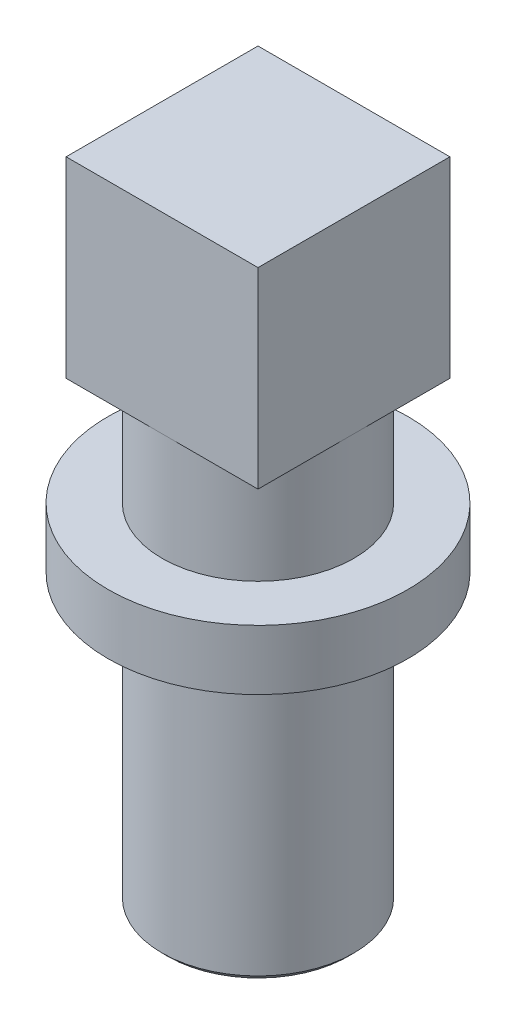
from build123d import *

# Parameters (mm, degrees)
SHANK_SKETCH_16_R             = 8
SHANK_16X24_DEPTH             = 24
SHANK_END_CHAMFER_0_5X45_SIZE = 0.5
COLLAR_SKETCH_25_R            = 12.5
COLLAR_25X5_DEPTH             = 5
NECK_SKETCH_16_R              = 8
NECK_16X9_DEPTH               = 9
SQUARE_HEAD_SKETCH_16X16_W    = 16
SQUARE_HEAD_SKETCH_16X16_H    = 16
SQUARE_HEAD_16X16X16_DEPTH    = 16


with BuildPart() as part:
    # Shank Sketch Ø16 → Shank Ø16x24 (new body)
    with BuildSketch(Plane(origin=(0, 0, 0), x_dir=(1, 0, 0), z_dir=(0, 1, 0))):
        with Locations(Location((0, 0, 0), (0, 0, 270))):
            Circle(SHANK_SKETCH_16_R)
    extrude(amount=SHANK_16X24_DEPTH)

    # Shank End Chamfer 0.5x45
    shank_end_chamfer_0_5x45_edges = [part.edges().sort_by_distance(p)[0] for p in [
        (0, 0, -8),
    ]]
    chamfer(shank_end_chamfer_0_5x45_edges, length=SHANK_END_CHAMFER_0_5X45_SIZE)

    # Collar Sketch Ø25 → Collar Ø25x5 (add)
    with BuildSketch(Plane(origin=(0, 24, 0), x_dir=(1, 0, 0), z_dir=(0, 1, 0))):
        with Locations(Location((0, 0, 0), (0, 0, 270))):
            Circle(COLLAR_SKETCH_25_R)
    extrude(amount=COLLAR_25X5_DEPTH)

    # Neck Sketch Ø16 → Neck Ø16x9 (add)
    with BuildSketch(Plane(origin=(0, 29, 0), x_dir=(1, 0, 0), z_dir=(0, 1, 0))):
        with Locations(Location((0, 0, 0), (0, 0, 270))):
            Circle(NECK_SKETCH_16_R)
    extrude(amount=NECK_16X9_DEPTH)

    # Square Head Sketch 16x16 → Square Head 16x16x16 (add)
    with BuildSketch(Plane(origin=(0, 38, 0), x_dir=(1, 0, 0), z_dir=(0, 1, 0))):
        Rectangle(SQUARE_HEAD_SKETCH_16X16_W, SQUARE_HEAD_SKETCH_16X16_H)
    extrude(amount=SQUARE_HEAD_16X16X16_DEPTH)


solid = part.part
